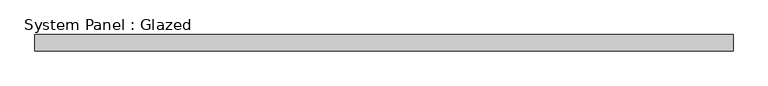
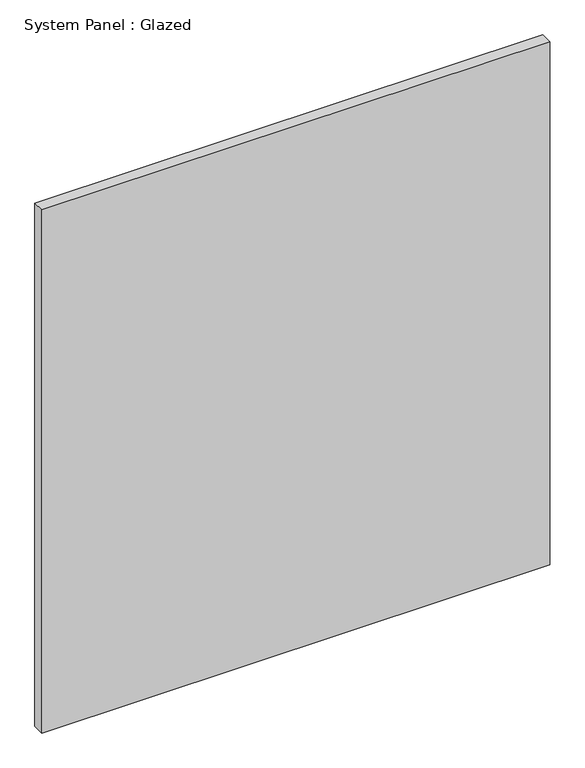
"""IFC4 building model written with IfcOpenShell, lengths in millimetres: plate geometry, System Panel : Glazed."""

from ifc_helpers import new_model, si_unit, origin, origin_with_axes, place, context, project, spatial, polyline, outline, extrude, source, transform, mapped, element, save


def system_panel_glazed_de674e10(model_context):
    return source(origin(), model_context, "Body", "SweptSolid", [
        extrude(outline(polyline([(550.3333332, 19.05), (-550.3333332, 19.05), (-550.3333332, 44.45), (550.3333332, 44.45), (550.3333332, 19.05)])), origin_with_axes(), (0.0, 0.0, 1.0), 1198.6188597),
    ])


if __name__ == "__main__":
    model = new_model("IFC4")
    model_context = context("Model", 3, world=origin())
    ifc_project = project(units=[si_unit("LENGTHUNIT", "METRE", prefix="MILLI")], contexts=[model_context])
    site = spatial("IfcSite", under=ifc_project)
    building = spatial("IfcBuilding", under=site)
    placement = place(None, origin())
    system_panel_glazed_shape = system_panel_glazed_de674e10(model_context)
    element("IfcPlate", 1, ObjectType="System Panel : Glazed", at=placement, inside=building, context=model_context, shape_type="MappedRepresentation", body=[
        mapped(system_panel_glazed_shape, transform((0.0, 0.0, 0.0), x_axis=(1.0, 0.0, 0.0), y_axis=(0.0, 1.0, 0.0), z_axis=(0.0, 0.0, 1.0))),
    ])
    save(model, "model.ifc")

# Revit data of these elements
# Type "System Panel : Glazed"
#   Construction Type Id = "GSP4R"
#   Analytic Construction = "1/8 in Pilkington single glazing"
#   Visual Light Transmittance = 0.9
#   Solar Heat Gain Coefficient = 0.86
#   Heat Transfer Coefficient (U) = 1.18115 BTU/(h·ft²·°F)
#   Define Thermal Properties by = 1
# Element 1 (IfcPlate, "System Panel : Glazed")
#   Materials on its faces: "Glass"
# Materials
#   "Glass": class "Glass", colour RGB 0 128 192, transparency 0.75, Description = "Soda Lime Glass", Cost = 0
